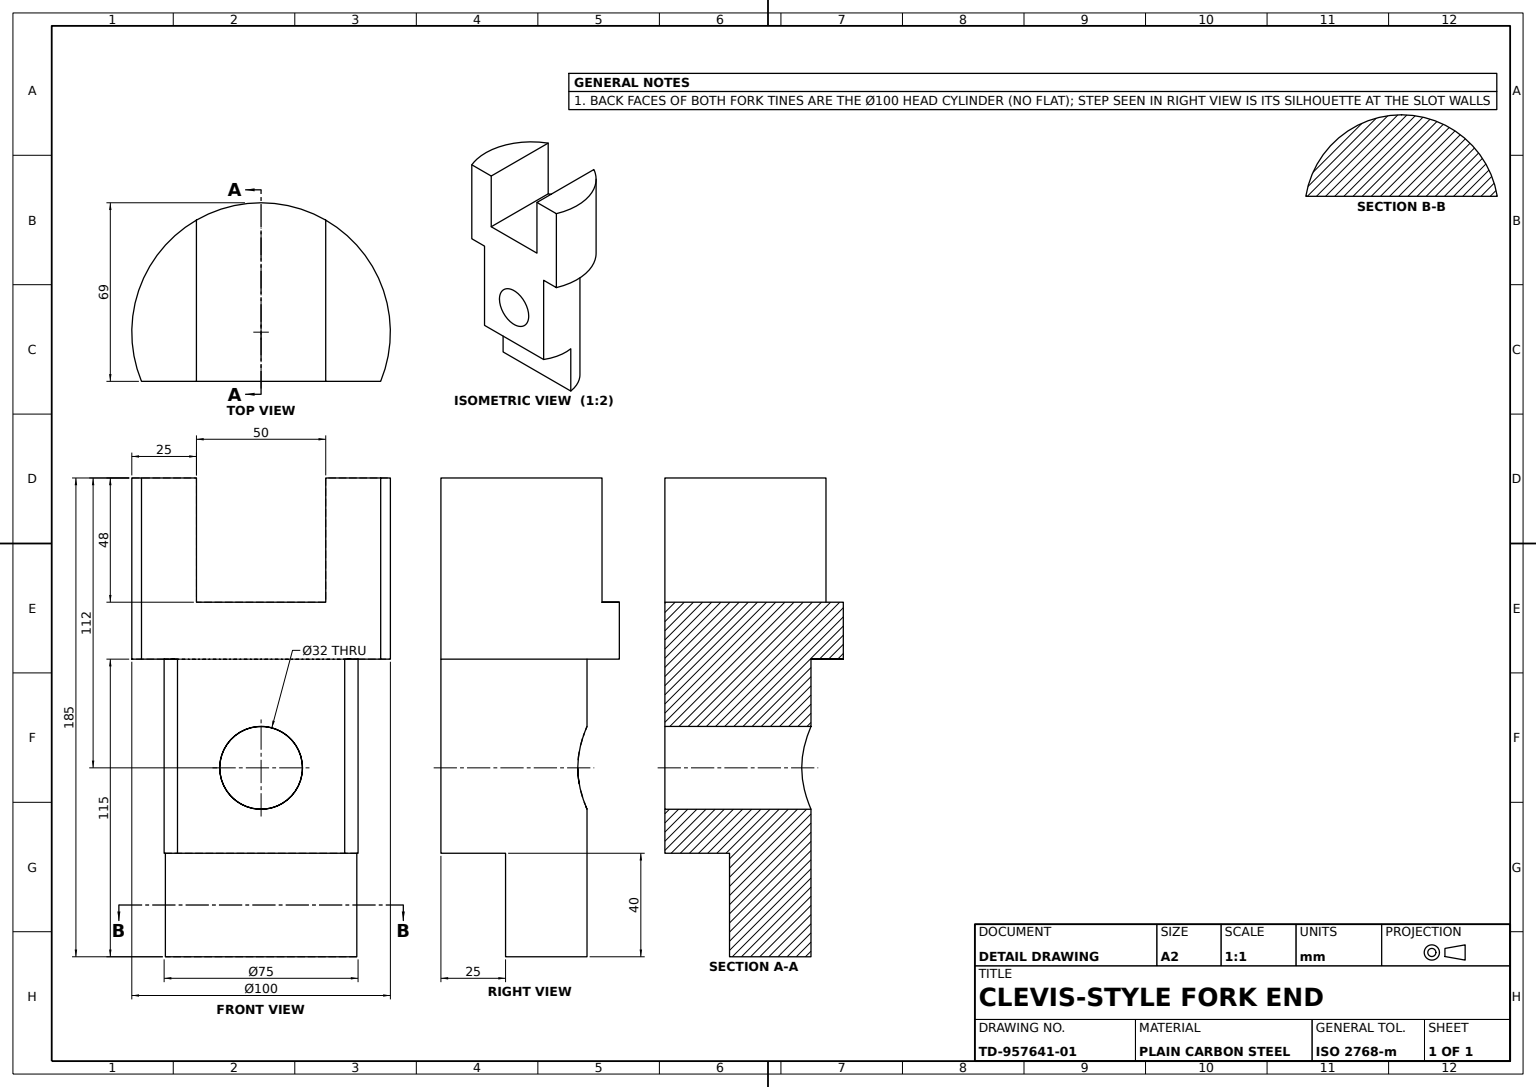
SolidWorks part; units mm, degrees
material "Plain Carbon Steel"
ref_plane "Front Plane" through (0, 0, 0) normal (0, 0, 1) x (1, 0, 0)
ref_plane "Top Plane" through (0, 0, 0) normal (0, 1, 0) x (1, 0, 0)
ref_plane "Right Plane" through (0, 0, 0) normal (1, 0, 0) x (0, 0, -1)
sketch "Shank Profile Ø75" plane through (0, 0, 0) normal (0, 1, 0) x (1, 0, 0)
  circle A0 centre (0, 0) radius 37.5
  dimension "D1" = 75
extrude "Shank Ø75" add sketch "Shank Profile Ø75" along normal blind 115
sketch "Head Profile Ø100" plane through (0, 115, 0) normal (0, 1, 0) x (1, 0, 0)
  circle A0 centre (0, 0) radius 50
  dimension "D1" = 100
extrude "Fork Head Ø100" add sketch "Head Profile Ø100" along normal blind 70
sketch "Flat Face Profile" plane through (0, 185, 0) normal (0, 1, 0) x (1, 0, 0)
  line L0 (-81.0321, -19) -> (77.1212, -19)
  line L1 (-81.0321, -19) -> (5.6316, -69.1557)
  line L2 (5.6316, -69.1557) -> (77.1212, -19)
  circle A0 centre (0, 0) radius 50 construction
  dimension "D1" = 19
  dimension "D2" = 5.6316
  dimension "D3" = 77.1212
  dimension "D4" = 81.0321
  dimension "D5" = 69.1557
extrude "Flat Face Cut" cut sketch "Flat Face Profile" against normal blind 230
sketch "Fork Slot Profile" plane through (0, 0, 19) normal (0, 0, 1) x (1, 0, 0)
  line L0 (46.2493, 185) -> (-46.2493, 185) construction
  line L1 (-25, 199.84) -> (25, 199.84)
  line L2 (-25, 199.84) -> (-25, 137)
  line L3 (-25, 137) -> (25, 137)
  line L4 (25, 199.84) -> (25, 137)
  line L5 (-46.2493, 115) -> (-46.2493, 185) construction
  circle A0 centre (0, 73) radius 16
  dimension "D6" = 32
  dimension "D1" = 50
  dimension "D2" = 48
  dimension "D3" = 25
  dimension "D4" = 46.2493
  dimension "D5" = 14.84
  dimension "D7" = 112
extrude "Fork Slot Cut" cut sketch "Fork Slot Profile" against normal blind 230
sketch "Cross Hole Profile" plane through (0, 0, 19) normal (0, 0, 1) x (1, 0, 0)
  line L0 (-37.5, 115) -> (-37.5, 0) construction
  line L1 (37.5, 0) -> (-37.5, 0)
  line L2 (37.5, 0) -> (37.5, 40)
  line L3 (37.5, 40) -> (-37.5, 40)
  line L4 (-37.5, 0) -> (-37.5, 40)
  dimension "D1" = 40
extrude "Cross Hole Cut" cut sketch "Cross Hole Profile" against normal blind 25
